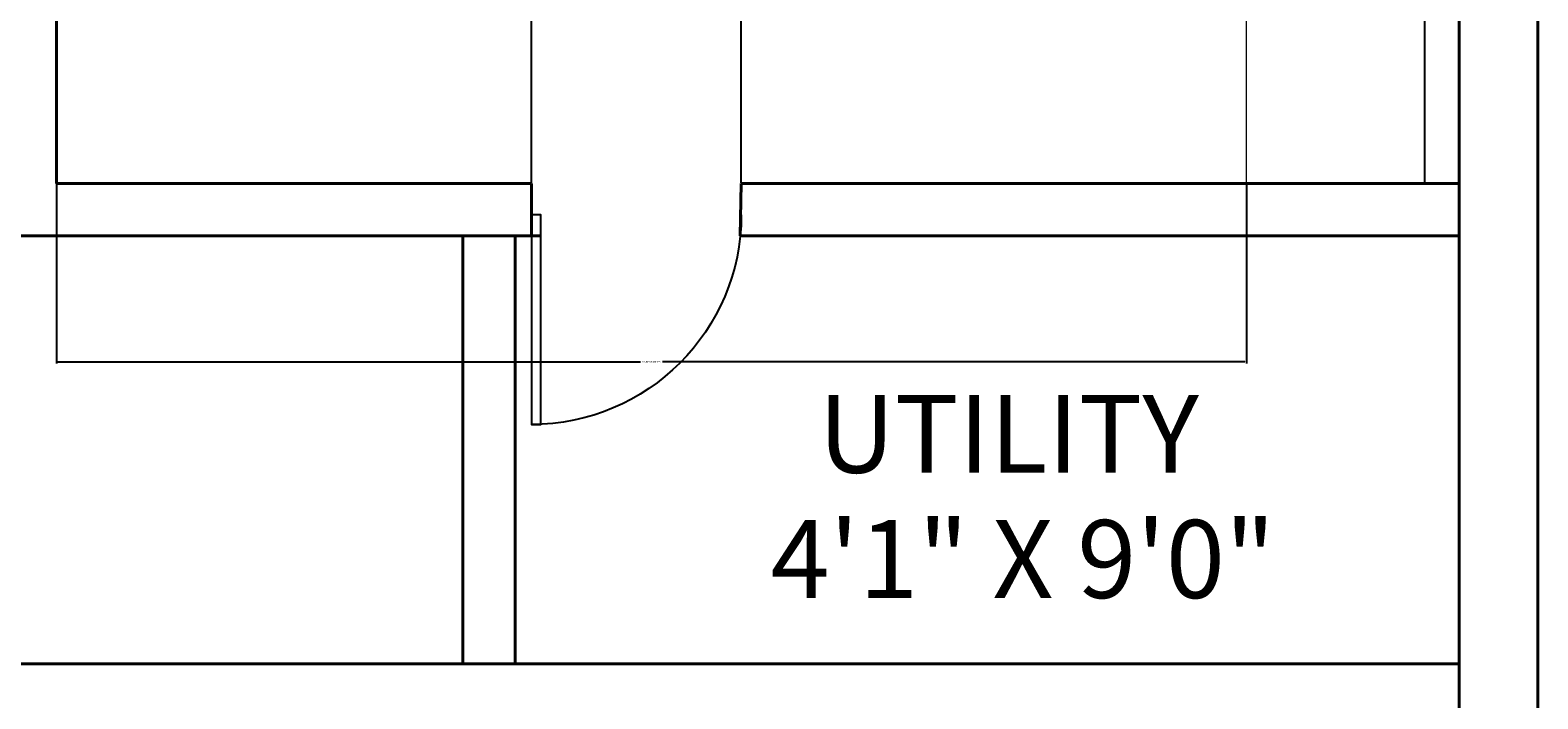
# Model space of a CAD drawing. Units: inches. Extents: x -46 to 1145, y -527 to 760.
# Tile 50 of 57: x 337 to 509, y 472 to 548. Entities that reach past the tile are written whole.
import ezdxf

# ---------------------------------------------------------------- set-up
doc = ezdxf.new("R2010")
doc.units = ezdxf.units.IN
doc.header["$MEASUREMENT"] = 0
for name, color, linetype, lineweight in [('A-ANNO-DIMS', 2, 'Continuous', 18), ('A-AREA-IDEN', 1, 'Continuous', 18), ('A-FLOR-CASE', 32, 'Continuous', 18), ('DOORS', 3, 'Continuous', 25), ('WALLS', 4, 'Continuous', 40)]:
    doc.layers.add(name, color=color, linetype=linetype, lineweight=lineweight)
doc.styles.get("Standard").update_dxf_attribs({"font": 'arial.ttf'})
doc.dimstyles.get("Standard").update_dxf_attribs({"dimtxt": 0.18, "dimasz": 0.18, "dimexe": 0.18, "dimexo": 0.0625, "dimgap": 0.09, "dimtad": 0, "dimtih": 1, "dimtoh": 1, "dimdec": 0, "dimzin": 0, "dimdsep": 46, "dimlunit": 3, "dimtxsty": 'Standard', "dimcen": 0.09, "dimadec": 0, "dimazin": 0, "dimtfac": 1, "dimtdec": 0, "dimtofl": 0, "dimtmove": 0, "dimatfit": 3, "dimfxl": 1, "dimtolj": 1, "dimtzin": 0, "dimarcsym": 0})

# ---------------------------------------------------------------- blocks, each defined once
blk = doc.blocks.new('*U2')
for p, q in [((0, 0), (0, -6)), ((40, 0), (40, -6))]:
    blk.add_line(p, q)
blk.add_lwpolyline([(0, 0), (0, 40), (1.75, 40), (1.75, 0)], close=True)
blk.add_arc((0, 0), 40, 0, 90)
blk = doc.blocks.new('KITCHEN-COUNTER-L')
for p, q in [((136.17, 96), (0, 96)), ((136.17, 24), (136.17, 96)), ((136.17, 0), (136.17, 24))]:
    blk.add_line(p, q)
blk = doc.blocks.new('*D682')
at = {"layer": 'A-ANNO-DIMS', "color": 0, "lineweight": -2, "transparency": 16777216}
for p, q in [((339.56, 530.46), (339.56, 509.91)), ((475.73, 530.46), (475.73, 509.91)), ((339.74, 510.09), (406.39, 510.09)), ((475.55, 510.09), (408.9, 510.09))]:
    blk.add_line(p, q, dxfattribs=at)
at = {"layer": 'A-ANNO-DIMS', "color": 0, "transparency": 16777216}
for points in [[(339.74, 510.12), (339.74, 510.06), (339.56, 510.09)], [(475.55, 510.12), (475.55, 510.06), (475.73, 510.09)]]:
    blk.add_solid(points, dxfattribs=at)
at = {"layer": 'Defpoints', "color": 0, "transparency": 16777216}
for p in [(339.56, 530.52), (475.73, 530.52), (475.73, 510.09)]:
    blk.add_point(p, dxfattribs=at)
at = {"layer": 'A-ANNO-DIMS', "color": 0, "transparency": 16777216, "insert": (407.65, 510.09), "char_height": 0.18, "attachment_point": 5}
blk.add_mtext('\\A1;COUNTER 136 TYP.', dxfattribs=at)
blk = doc.blocks.new('*D683')
at = {"layer": 'A-ANNO-DIMS', "color": 0, "lineweight": -2, "transparency": 16777216}
for p, q in [((475.79, 626.52), (496.33, 626.52)), ((496.15, 626.34), (496.15, 578.7)), ((496.15, 530.7), (496.15, 578.34)), ((475.79, 530.52), (496.33, 530.52))]:
    blk.add_line(p, q, dxfattribs=at)
at = {"layer": 'A-ANNO-DIMS', "color": 0, "transparency": 16777216}
for points in [[(496.12, 626.34), (496.18, 626.34), (496.15, 626.52)], [(496.12, 530.7), (496.18, 530.7), (496.15, 530.52)]]:
    blk.add_solid(points, dxfattribs=at)
at = {"layer": 'Defpoints', "color": 0, "transparency": 16777216}
for p in [(475.73, 626.52), (496.15, 626.52), (475.73, 530.52)]:
    blk.add_point(p, dxfattribs=at)
at = {"layer": 'A-ANNO-DIMS', "color": 0, "transparency": 16777216, "insert": (496.15, 578.52), "char_height": 0.18, "attachment_point": 5}
blk.add_mtext('\\A1;96 TYP.', dxfattribs=at)
blk = doc.blocks.new('*D699')
at = {"layer": 'A-ANNO-DIMS', "color": 0, "lineweight": -2, "transparency": 16777216}
for p, q in [((393.93, 530.58), (393.93, 759.67)), ((394.11, 759.49), (405.71, 759.49)), ((417.75, 759.49), (406.15, 759.49)), ((417.93, 530.58), (417.93, 759.67))]:
    blk.add_line(p, q, dxfattribs=at)
at = {"layer": 'A-ANNO-DIMS', "color": 0, "transparency": 16777216}
for points in [[(394.11, 759.52), (394.11, 759.46), (393.93, 759.49)], [(417.75, 759.52), (417.75, 759.46), (417.93, 759.49)]]:
    blk.add_solid(points, dxfattribs=at)
at = {"layer": 'Defpoints', "color": 0, "transparency": 16777216}
for p in [(417.93, 759.49), (393.93, 530.52), (417.93, 530.52)]:
    blk.add_point(p, dxfattribs=at)
at = {"layer": 'A-ANNO-DIMS', "color": 0, "transparency": 16777216, "insert": (405.93, 759.49), "char_height": 0.18, "attachment_point": 5}
blk.add_mtext('\\A1;24', dxfattribs=at)

msp = doc.modelspace()

# ---------------------------------------------------------------- linework, layer by layer
at = {"layer": 'WALLS'}
for p, q in [((509.0637, 659.5176), (509.0637, 221.5176)), ((339.5637, 650.5176), (339.5637, 530.5176)), ((500.0637, 650.5176), (500.0637, 524.5176)), ((339.5637, 530.5176), (393.9282, 530.5176)), ((393.9282, 530.5176), (393.9282, 524.5176)), ((417.9282, 530.5176), (417.8079, 524.5176)), ((417.9282, 530.5176), (500.0637, 530.5176)), ((333.5637, 524.5176), (394.9782, 524.5176)), ((386.0637, 475.5176), (386.0637, 524.5176)), ((392.0637, 475.5176), (392.0637, 524.5176)), ((417.8079, 524.5176), (500.0637, 524.5176)), ((500.0637, 475.5176), (500.0637, 524.5176)), ((333.5637, 475.5176), (500.0637, 475.5176)), ((500.0637, 475.5176), (500.0637, 469.5176))]:
    msp.add_line(p, q, dxfattribs=at)

# ---------------------------------------------------------------- block references
at = {"layer": 'A-FLOR-CASE'}
msp.add_blockref('KITCHEN-COUNTER-L', (339.564, 530.518), dxfattribs=at)
at = {"layer": 'DOORS', "xscale": -0.6, "yscale": 0.6, "zscale": 0.6, "rotation": 180}
msp.add_blockref('*U2', (393.9282, 526.9176), dxfattribs=at)

# ---------------------------------------------------------------- texts
at = {"layer": 'A-AREA-IDEN'}
for s, height, p in [('   UTILITY', 8.92326, (418.5384, 497.3824)), (' 4\'1" X 9\'0"', 8.923264, (418.5384, 483.0479))]:
    msp.add_text(s, height=height, dxfattribs=at).set_placement(p)

# ---------------------------------------------------------------- dimensions: what is measured, and where the dimension line sits
at = {"layer": 'A-ANNO-DIMS'}
dim = msp.add_linear_dim(base=(417.9282, 759.4886), p1=(393.9282, 530.5176), p2=(417.9282, 530.5176), dimstyle='Standard', override={"dimdec": 0, "dimlfac": 1, "dimrnd": 0, "dimzin": 0, "dimdsep": 46, "dimlunit": 2}, dxfattribs=at)
dim.commit()
dim.dimension.update_dxf_attribs({"geometry": '*D699', "text_midpoint": (405.9282, 759.4886)})
dim = msp.add_linear_dim(base=(496.1541, 626.5176), p1=(475.7292, 530.5176), p2=(475.7292, 626.5176), angle=90, text='<> TYP.', dimstyle='Standard', override={"dimdec": 0, "dimlfac": 1, "dimrnd": 0, "dimzin": 0, "dimdsep": 46, "dimlunit": 2}, dxfattribs=at)
dim.commit()
dim.dimension.update_dxf_attribs({"geometry": '*D683', "text_midpoint": (496.1541, 578.5176)})
dim = msp.add_linear_dim(base=(475.7292, 510.0927), p1=(339.5637, 530.5176), p2=(475.7292, 530.5176), text='COUNTER <> TYP.', dimstyle='Standard', override={"dimdec": 0, "dimlfac": 1, "dimrnd": 0, "dimzin": 0, "dimdsep": 46, "dimlunit": 2}, dxfattribs=at)
dim.commit()
dim.dimension.update_dxf_attribs({"geometry": '*D682', "text_midpoint": (407.6465, 510.0927)})

doc.saveas('drawing.dxf')
